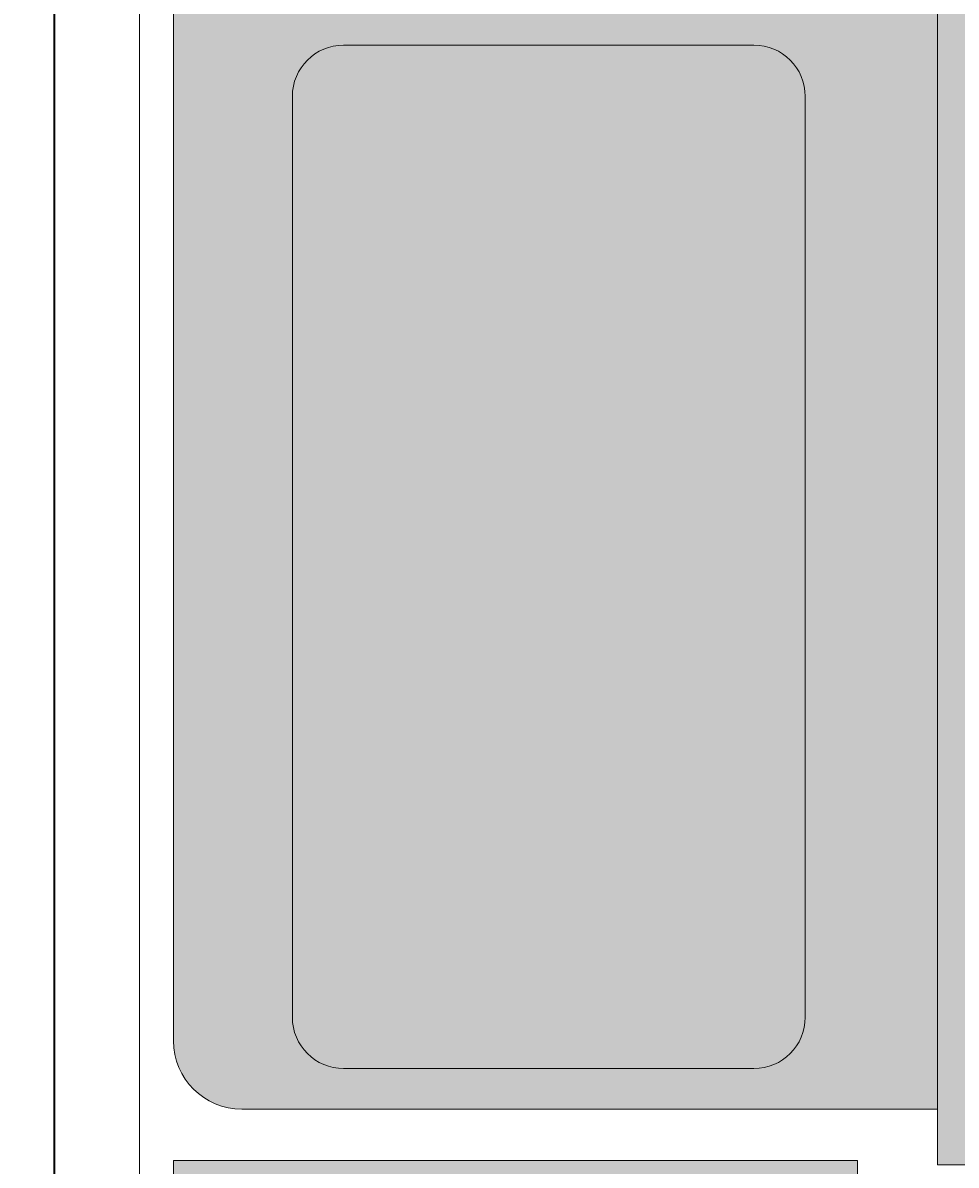
# Model space of a CAD drawing. Units: millimetres. Extents: x 27017497 to 27018854, y 7058029 to 7059154.
# Tile 81 of 91: x 27018319 to 27018341, y 7058503 to 7058530. Entities that reach past the tile are written whole.
import ezdxf

# ---------------------------------------------------------------- set-up
doc = ezdxf.new("R2010")
doc.units = ezdxf.units.MM
for name, color, linetype, lineweight in [('A-ANNO-DIMS', 2, 'Continuous', 18), ('A-FURN', 8, 'Continuous', 18), ('A-WALL', 7, 'Continuous', 35)]:
    doc.layers.add(name, color=color, linetype=linetype, lineweight=lineweight)
doc.layers.add('A-FURN-PATT', color=177, linetype='Continuous', lineweight=13, true_color=0x293189)
doc.styles.get("Standard").update_dxf_attribs({"font": 'arial.ttf'})
doc.dimstyles.get("Standard").update_dxf_attribs({"dimtxt": 0.18, "dimasz": 0.18, "dimexe": 0.18, "dimexo": 0.0625, "dimgap": 0.09, "dimtad": 0, "dimtih": 1, "dimtoh": 1, "dimdec": 4, "dimzin": 0, "dimdsep": 46, "dimtxsty": 'Standard', "dimcen": 0.09, "dimadec": 0, "dimazin": 0, "dimtfac": 1, "dimtdec": 4, "dimtofl": 0, "dimtmove": 0, "dimatfit": 3, "dimfxl": 1, "dimtolj": 1, "dimtzin": 0, "dimarcsym": 0})

# ---------------------------------------------------------------- blocks, each defined once
blk = doc.blocks.new('CAMMAT')
for p, q in [((1.27313, 0), (-1.27313, 0)), ((1.27313, -0.05), (-1.27313, -0.05)), ((0.61, -0.07), (-0.61, -0.07)), ((0.68, -0.07), (0.68, -0.47)), ((0.68, -0.07), (1.18, -0.07)), ((0.65, -0.11), (0.65, -0.51693)), ((0.59619, -0.1395), (0.05741, -0.1395)), ((0.02741, -0.1695), (0.02741, -0.4095)), ((0.62619, -0.1695), (0.62619, -0.4095)), ((0.59619, -0.4395), (0.05741, -0.4395)), ((0.68, -0.47), (1.18, -0.47)), ((-0.6904, -0.51693), (0.68256, -0.51693)), ((0.68256, -0.51693), (0.68256, -0.76028))]:
    blk.add_line(p, q)
for centre, radius, start, end in [((0.61, -0.11), 0.04, 0, 90), ((0.05741, -0.1695), 0.03, 90, 180), ((0.59619, -0.1695), 0.03, 360, 90), ((0.05741, -0.4095), 0.03, 180, 270), ((0.59619, -0.4095), 0.03, 270, 360)]:
    blk.add_arc(centre, radius, start, end)
blk = doc.blocks.new('*D48')
at = {"layer": 'A-ANNO-DIMS', "color": 0, "lineweight": -2, "transparency": 16777216}
for p, q in [((27018463.498, 7058622.912), (27017497.536, 7058622.912)), ((27017497.716, 7058622.732), (27017497.716, 7058357.753)), ((27017497.716, 7058092.41), (27017497.716, 7058357.389)), ((27018555.129, 7058092.23), (27017497.536, 7058092.23))]:
    blk.add_line(p, q, dxfattribs=at)
at = {"layer": 'A-ANNO-DIMS', "color": 0, "transparency": 16777216}
for points in [[(27017497.686, 7058622.732), (27017497.746, 7058622.732), (27017497.716, 7058622.912)], [(27017497.686, 7058092.41), (27017497.746, 7058092.41), (27017497.716, 7058092.23)]]:
    blk.add_solid(points, dxfattribs=at)
at = {"layer": 'Defpoints', "color": 0, "transparency": 16777216}
for p in [(27018463.561, 7058622.912), (27017497.716, 7058092.23), (27018555.192, 7058092.23)]:
    blk.add_point(p, dxfattribs=at)
at = {"layer": 'A-ANNO-DIMS', "color": 0, "transparency": 16777216, "insert": (27017497.716, 7058357.571), "char_height": 0.18, "attachment_point": 5}
blk.add_mtext('\\A1;530.7', dxfattribs=at)
blk = doc.blocks.new('*D50')
at = {"layer": 'A-ANNO-DIMS', "color": 0, "lineweight": -2, "transparency": 16777216}
for p, q in [((27018223.668, 7058580.912), (27018854.236, 7058580.912)), ((27018854.056, 7058580.732), (27018854.056, 7058511.344)), ((27018854.056, 7058441.592), (27018854.056, 7058510.98)), ((27018223.668, 7058441.412), (27018854.236, 7058441.412))]:
    blk.add_line(p, q, dxfattribs=at)
at = {"layer": 'A-ANNO-DIMS', "color": 0, "transparency": 16777216}
for points in [[(27018854.026, 7058580.732), (27018854.086, 7058580.732), (27018854.056, 7058580.912)], [(27018854.026, 7058441.592), (27018854.086, 7058441.592), (27018854.056, 7058441.412)]]:
    blk.add_solid(points, dxfattribs=at)
at = {"layer": 'Defpoints', "color": 0, "transparency": 16777216}
for p in [(27018223.606, 7058580.912), (27018223.606, 7058441.412), (27018854.056, 7058441.412)]:
    blk.add_point(p, dxfattribs=at)
at = {"layer": 'A-ANNO-DIMS', "color": 0, "transparency": 16777216, "insert": (27018854.056, 7058511.162), "char_height": 0.18, "attachment_point": 5}
blk.add_mtext('\\A1;139.5', dxfattribs=at)

msp = doc.modelspace()

# ---------------------------------------------------------------- hatches: boundary and pattern name
at = {"layer": 'A-FURN-PATT'}
h = msp.add_hatch(color=256, dxfattribs=at)
h.dxf.hatch_style = 1
h.paths.add_polyline_path([(27018398.067, 7058554.497, 0.414214), (27018396.474, 7058556.09), (27018352.018, 7058556.09), (27018352.202, 7058552.834), (27018352.581, 7058547.929), (27018353.082, 7058544.346), (27018353.818, 7058541.828), (27018354.899, 7058540.115), (27018356.437, 7058538.948), (27018358.543, 7058538.068), (27018361.329, 7058537.215), (27018358.524, 7058536.613), (27018356.284, 7058536.07), (27018354.381, 7058535.48), (27018352.588, 7058534.736), (27018350.68, 7058533.729), (27018348.431, 7058532.354), (27018345.612, 7058530.503), (27018341.998, 7058528.068), (27018345.612, 7058525.633), (27018348.431, 7058523.782), (27018350.68, 7058522.407), (27018352.588, 7058521.4), (27018354.381, 7058520.656), (27018356.284, 7058520.066), (27018358.524, 7058519.523), (27018361.329, 7058518.92), (27018358.543, 7058518.068), (27018356.437, 7058517.188), (27018354.899, 7058516.021), (27018353.818, 7058514.308), (27018353.082, 7058511.79), (27018352.581, 7058508.207), (27018352.28, 7058504.311), (27018396.474, 7058504.311, 0.414214), (27018398.067, 7058505.904)])
h.paths.add_polyline_path([(27018356.437, 7058538.948), (27018354.899, 7058540.115), (27018353.818, 7058541.828), (27018353.082, 7058544.346), (27018352.581, 7058547.929), (27018352.202, 7058552.834), (27018351.835, 7058559.322), (27018341.998, 7058528.068), (27018345.612, 7058530.503), (27018348.431, 7058532.354), (27018350.68, 7058533.729), (27018352.588, 7058534.736), (27018354.381, 7058535.48), (27018356.284, 7058536.07), (27018358.524, 7058536.613), (27018361.329, 7058537.215), (27018358.543, 7058538.068)])
h.paths.add_polyline_path([(27018358.543, 7058518.068), (27018361.329, 7058518.92), (27018358.524, 7058519.523), (27018356.284, 7058520.066), (27018354.381, 7058520.656), (27018352.588, 7058521.4), (27018350.68, 7058522.407), (27018348.431, 7058523.782), (27018345.612, 7058525.633), (27018341.998, 7058528.068), (27018351.835, 7058496.813), (27018352.202, 7058503.301), (27018352.581, 7058508.207), (27018353.082, 7058511.79), (27018353.818, 7058514.308), (27018354.899, 7058516.021), (27018356.437, 7058517.188)])
h.paths.add_polyline_path([(27018351.324, 7058557.699), (27018340.191, 7058557.699), (27018340.191, 7058503.014), (27018349.884, 7058503.014), (27018341.998, 7058528.068)])
h.paths.add_polyline_path([(27018340.191, 7058556.09), (27018323.983, 7058556.09, 0.414214), (27018322.39, 7058554.497), (27018322.39, 7058505.904, 0.414214), (27018323.983, 7058504.311), (27018340.191, 7058504.311)])
h.paths.add_polyline_path([(27018337.107, 7058532.051, -0.414214), (27018335.912, 7058530.856), (27018326.353, 7058530.856, -0.414214), (27018325.158, 7058532.051), (27018325.158, 7058553.51, -0.414214), (27018326.353, 7058554.705), (27018335.912, 7058554.705, -0.414214), (27018337.107, 7058553.51)], flags=0)
h.paths.add_polyline_path([(27018337.107, 7058527.914), (27018337.107, 7058506.454, -0.414214), (27018335.912, 7058505.259), (27018326.353, 7058505.259, -0.414214), (27018325.158, 7058506.454), (27018325.158, 7058527.914, -0.414214), (27018326.353, 7058529.109), (27018335.912, 7058529.109, -0.414214)], flags=0)
h.paths.add_polyline_path([(27018338.322, 7058577.2), (27018322.39, 7058577.2), (27018322.39, 7058557.285), (27018338.322, 7058557.285)])
h.paths.add_polyline_path([(27018323.748, 7058567.284, -1), (27018335.697, 7058567.284, -1)], flags=16)
h.paths.add_polyline_path([(27018326.023, 7058567.284, -1), (27018333.423, 7058567.284, -1)], flags=0)
h.paths.add_polyline_path([(27018338.322, 7058503.116), (27018322.39, 7058503.116), (27018322.39, 7058483.201), (27018338.322, 7058483.201)])
h.paths.add_polyline_path([(27018335.697, 7058493.391, -1), (27018323.748, 7058493.391, -1)], flags=16)
h.paths.add_polyline_path([(27018333.423, 7058493.391, -1), (27018326.023, 7058493.391, -1)], flags=0)
h.paths.add_polyline_path([(27018337.107, 7058527.914, 0.414214), (27018335.912, 7058529.109), (27018326.353, 7058529.109, 0.414214), (27018325.158, 7058527.914), (27018325.158, 7058506.454, 0.414214), (27018326.353, 7058505.259), (27018335.912, 7058505.259, 0.414214), (27018337.107, 7058506.454)], flags=16)
h.paths.add_polyline_path([(27018337.107, 7058553.51, 0.414214), (27018335.912, 7058554.705), (27018326.353, 7058554.705, 0.414214), (27018325.158, 7058553.51), (27018325.158, 7058532.051, 0.414214), (27018326.353, 7058530.856), (27018335.912, 7058530.856, 0.414214), (27018337.107, 7058532.051)], flags=16)
h = msp.add_hatch(color=256, dxfattribs=at)
h.dxf.hatch_style = 1
h.paths.add_polyline_path([(27018337.107, 7058553.51, 0.414214), (27018335.912, 7058554.705), (27018326.353, 7058554.705, 0.414214), (27018325.158, 7058553.51), (27018325.158, 7058532.051, 0.414214), (27018326.353, 7058530.856), (27018335.912, 7058530.856, 0.414214), (27018337.107, 7058532.051)])
h.paths.add_polyline_path([(27018337.107, 7058527.914, 0.414214), (27018335.912, 7058529.109), (27018326.353, 7058529.109, 0.414214), (27018325.158, 7058527.914), (27018325.158, 7058506.454, 0.414214), (27018326.353, 7058505.259), (27018335.912, 7058505.259, 0.414214), (27018337.107, 7058506.454)])

# ---------------------------------------------------------------- linework, layer by layer
at = {"layer": 'A-WALL'}
msp.add_line((27018319.606, 7058580.912), (27018319.606, 7058412.636), dxfattribs=at)

# ---------------------------------------------------------------- block references
at = {"layer": 'A-FURN', "xscale": -39.82996475819422, "yscale": 39.82996475819422, "zscale": 39.82996475819422, "rotation": 90}
msp.add_blockref('CAMMAT', (27018319.602, 7058530.2), dxfattribs=at)

# ---------------------------------------------------------------- dimensions: what is measured, and where the dimension line sits
at = {"layer": 'A-ANNO-DIMS'}
for base, p1, p2, picture, middle in [((27017497.716, 7058092.23), (27018463.561, 7058622.912), (27018555.192, 7058092.23), '*D48', (27017497.716, 7058357.571)), ((27018854.056, 7058441.412), (27018223.606, 7058580.912), (27018223.606, 7058441.412), '*D50', (27018854.056, 7058511.162))]:
    dim = msp.add_linear_dim(base=base, p1=p1, p2=p2, angle=90, dimstyle='Standard', override={"dimdec": 1, "dimlfac": 1, "dimrnd": 0, "dimzin": 0, "dimdsep": 46, "dimlunit": 2}, dxfattribs=at)
    dim.commit()
    dim.dimension.update_dxf_attribs({"geometry": picture, "text_midpoint": middle})

doc.saveas('drawing.dxf')
